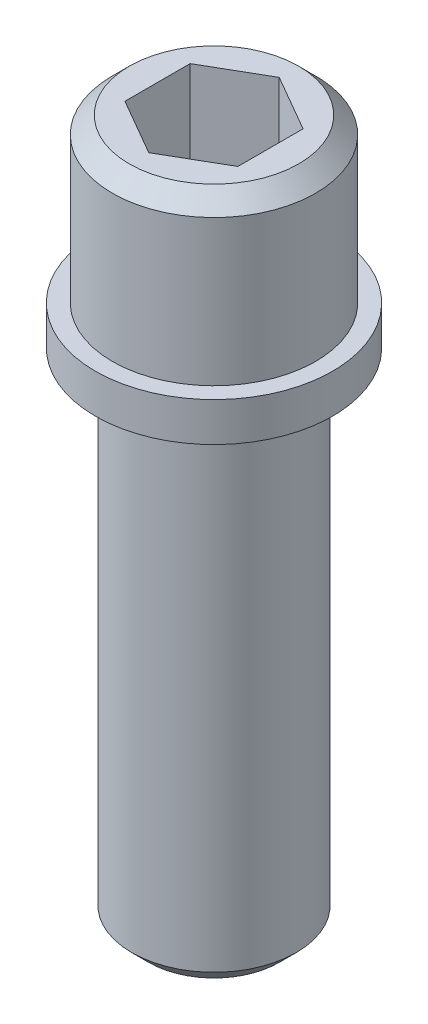
from build123d import *

# Parameters (mm, degrees)
SHANK_SKETCH_9_7_R            = 4.85
SHANK_9_7X29_5_DEPTH          = 29.5
FLANGE_SKETCH_17_3_R          = 7
FLANGE_17_3X2_3_DEPTH         = 2.3
HEAD_SKETCH_12_R              = 6
HEAD_12X9_6_DEPTH             = 9.6
HEX_SOCKET_7_7X9_6_DEEP_DEPTH = 9.6
HEAD_TOP_CHAMFER_1X45_SIZE    = 1
SHANK_END_CHAMFER_1X45_SIZE   = 1


with BuildPart() as part:
    # Shank Sketch Ø9.7 → Shank Ø9.7x29.5 (new body)
    with BuildSketch(Plane(origin=(0, 0, 0), x_dir=(1, 0, 0), z_dir=(0, 1, 0))):
        with Locations(Location((0, 0, 0), (0, 0, 270))):
            Circle(SHANK_SKETCH_9_7_R)
    extrude(amount=SHANK_9_7X29_5_DEPTH)

    # Flange Sketch Ø17.3 → Flange Ø17.3x2.3 (add)
    with BuildSketch(Plane(origin=(0, 29.5, 0), x_dir=(1, 0, 0), z_dir=(0, 1, 0))):
        with Locations(Location((0, 0, 0), (0, 0, 270))):
            Circle(FLANGE_SKETCH_17_3_R)
    extrude(amount=FLANGE_17_3X2_3_DEPTH)

    # Head Sketch Ø12 → Head Ø12x9.6 (add)
    with BuildSketch(Plane(origin=(0, 31.8, 0), x_dir=(1, 0, 0), z_dir=(0, 1, 0))):
        with Locations(Location((0, 0, 0), (0, 0, 270))):
            Circle(HEAD_SKETCH_12_R)
    extrude(amount=HEAD_12X9_6_DEPTH)

    # Hex Socket Sketch 7.7 → Hex Socket 7.7x9.6 Deep (cut)
    with BuildSketch(Plane(origin=(0, 41.4, 0), x_dir=(1, 0, 0), z_dir=(0, 1, 0))):
        Polygon((0, 3.85), (-3.334197805, 1.925), (-3.334197805, -1.925), (0, -3.85), (3.334197805, -1.925), (3.334197805, 1.925), align=None)
    extrude(amount=-HEX_SOCKET_7_7X9_6_DEEP_DEPTH, mode=Mode.SUBTRACT)

    # Head Top Chamfer 1x45
    head_top_chamfer_1x45_edges = [part.edges().sort_by_distance(p)[0] for p in [
        (0, 41.4, -6),
    ]]
    chamfer(head_top_chamfer_1x45_edges, length=HEAD_TOP_CHAMFER_1X45_SIZE)

    # Shank End Chamfer 1x45
    shank_end_chamfer_1x45_edges = [part.edges().sort_by_distance(p)[0] for p in [
        (0, 0, -4.85),
    ]]
    chamfer(shank_end_chamfer_1x45_edges, length=SHANK_END_CHAMFER_1X45_SIZE)


solid = part.part
